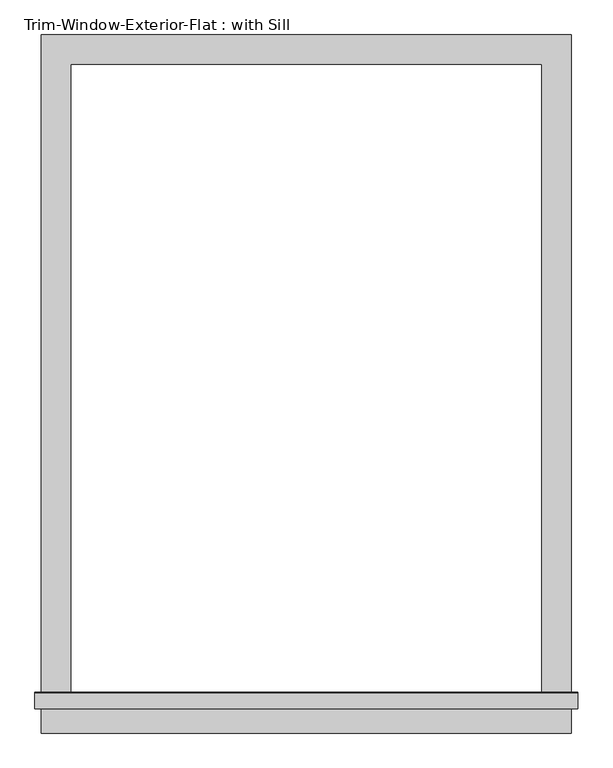
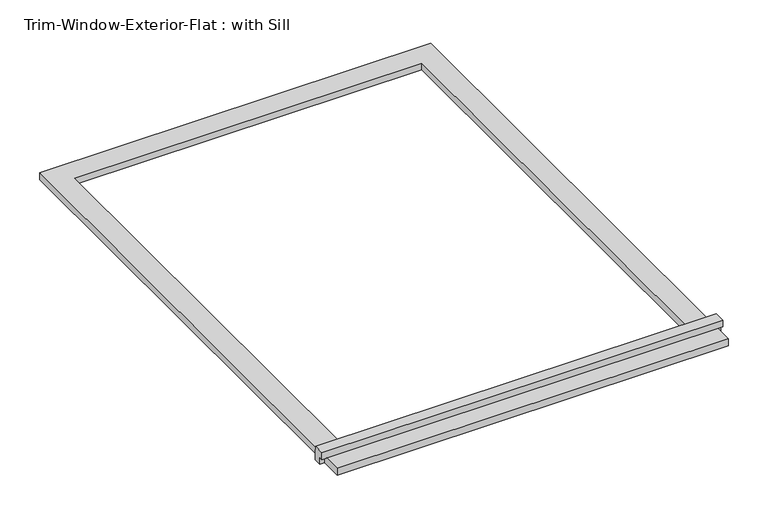
"""IFC4 building model written with IfcOpenShell, lengths in millimetres: proxy geometry, Trim-Window-Exterior-Flat : with Sill."""

from ifc_helpers import new_model, si_unit, frame, origin, origin_with_axes, place, context, project, spatial, polyline, outline, extrude, source, transform, mapped, element, save


def trim_window_exterior_flat_with_sill_e4b28ec3(model_context):
    return source(origin(), model_context, "Body", "SweptSolid", [
        extrude(outline(polyline([(514.35, -1241.3823709), (514.35, -1298.5323709), (-514.35, -1298.5323709), (-514.35, -1241.3823709), (514.35, -1241.3823709)])), origin_with_axes(), (0.0, 0.0, 1.0), 19.05),
        extrude(outline(polyline([(-1250.95, 38.1), (-1221.6580645, 38.1), (-1219.2, 19.05), (-1219.2, 0.0), (-1241.3823709, 0.0), (-1241.3823709, 19.05), (-1250.95, 19.05), (-1250.95, 38.1)])), frame((-527.05, 0.0, 0.0), z_axis=(1.0, 0.0, 0.0), x_axis=(0.0, 1.0, 0.0)), (0.0, 0.0, 1.0), 1054.1),
        extrude(outline(polyline([(-514.35, 57.15), (514.35, 57.15), (514.35, -1219.2), (457.2, -1219.2), (457.2, 0.0), (-457.2, 0.0), (-457.2, -1219.2), (-514.35, -1219.2), (-514.35, 57.15)])), origin_with_axes(), (0.0, 0.0, 1.0), 19.05),
    ])


if __name__ == "__main__":
    model = new_model("IFC4")
    model_context = context("Model", 3, world=origin())
    ifc_project = project(units=[si_unit("LENGTHUNIT", "METRE", prefix="MILLI")], contexts=[model_context])
    site = spatial("IfcSite", under=ifc_project)
    building = spatial("IfcBuilding", under=site)
    placement = place(None, origin())
    trim_window_exterior_flat_with_sill_shape = trim_window_exterior_flat_with_sill_e4b28ec3(model_context)
    element("IfcBuildingElementProxy", 1, Name="Trim-Window-Exterior-Flat : with Sill", ObjectType="Trim-Window-Exterior-Flat : with Sill", at=placement, inside=building, context=model_context, shape_type="MappedRepresentation", body=[
        mapped(trim_window_exterior_flat_with_sill_shape, transform((0.0, 0.0, 0.0), x_axis=(1.0, 0.0, 0.0), y_axis=(0.0, 1.0, 0.0), z_axis=(0.0, 0.0, 1.0))),
    ])
    save(model, "model.ifc")

# Revit data of these elements
# Type "Trim-Window-Exterior-Flat : with Sill"
#   Trim Width = 0' - 2 1/4"
#   Trim Thickness_Picture Frame = 0' - 1 1/4"
#   Trim Thickness_with Sill = 0' - 0 3/4"
#   Sill Thickness = 0' - 1 1/4"
#   Opening Width [instance default] = 2' - 0"
#   Opening Height [instance default] = 3' - 0"
#   Default Elevation = 4' - 0"
#   Sill = yes
#   Picture Frame = no
#   Trim Material [instance default] = none
# Element 1 (IfcBuildingElementProxy, "Trim-Window-Exterior-Flat : with Sill")
#   Opening Width = 3' - 0"
#   Opening Height = 4' - 0"
